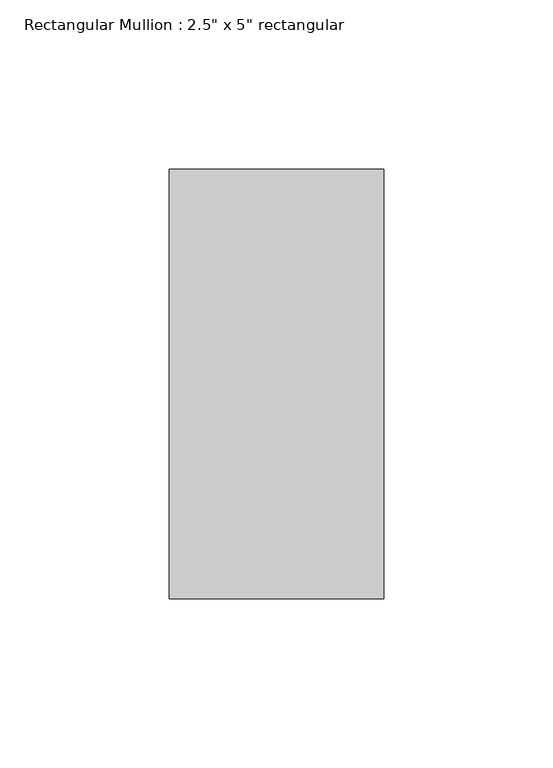
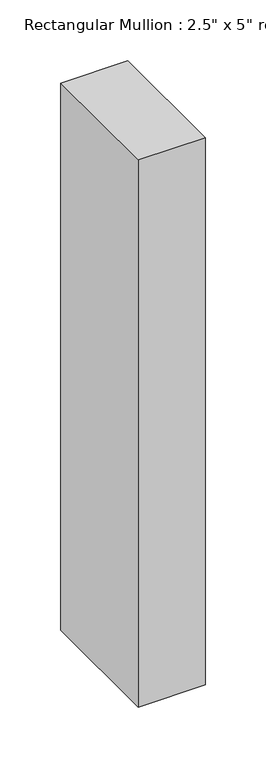
"""IFC4 building model written with IfcOpenShell, lengths in millimetres: member geometry."""

from ifc_helpers import new_model, si_unit, frame, origin, place, context, project, spatial, polyline, outline, extrude, source, transform, mapped, element, save


def member_f3803a17(model_context):
    return source(origin(), model_context, "Body", "SweptSolid", [
        extrude(outline(polyline([(31.75, 63.5), (31.75, -63.5), (-31.75, -63.5), (-31.75, 63.5), (31.75, 63.5)])), frame((0.0, 0.0, -549.036674), z_axis=(0.0, 0.0, 1.0), x_axis=(1.0, 0.0, 0.0)), (0.0, 0.0, 1.0), 549.036674),
    ])


if __name__ == "__main__":
    model = new_model("IFC4")
    model_context = context("Model", 3, world=origin())
    ifc_project = project(units=[si_unit("LENGTHUNIT", "METRE", prefix="MILLI")], contexts=[model_context])
    site = spatial("IfcSite", under=ifc_project)
    building = spatial("IfcBuilding", under=site)
    placement = place(None, origin())
    member_shape = member_f3803a17(model_context)
    element("IfcMember", 1, ObjectType="Rectangular Mullion : 2.5\" x 5\" rectangular", at=placement, inside=building, context=model_context, shape_type="MappedRepresentation", body=[
        mapped(member_shape, transform((0.0, 0.0, 0.0), x_axis=(1.0, 0.0, 0.0), y_axis=(0.0, 1.0, 0.0), z_axis=(0.0, 0.0, 1.0))),
    ])
    save(model, "model.ifc")

# Revit data of these elements
# Type "Rectangular Mullion : 2.5\" x 5\" rectangular"
#   built-in parameter 1007304 = 0.416667 (stored number, unit not read)
#   built-in parameter 1007301 = 0.104167 (stored number, unit not read)
#   built-in parameter 1007300 = 0.104167 (stored number, unit not read)
# Element 1 (IfcMember, "Rectangular Mullion : 2.5\" x 5\" rectangular")
#   Materials on its faces: "Aluminum"
# Materials
#   "Aluminum": class "Metal", colour RGB 247 247 247, transparency 0, Description = "Aluminum 6061", Cost = 0
